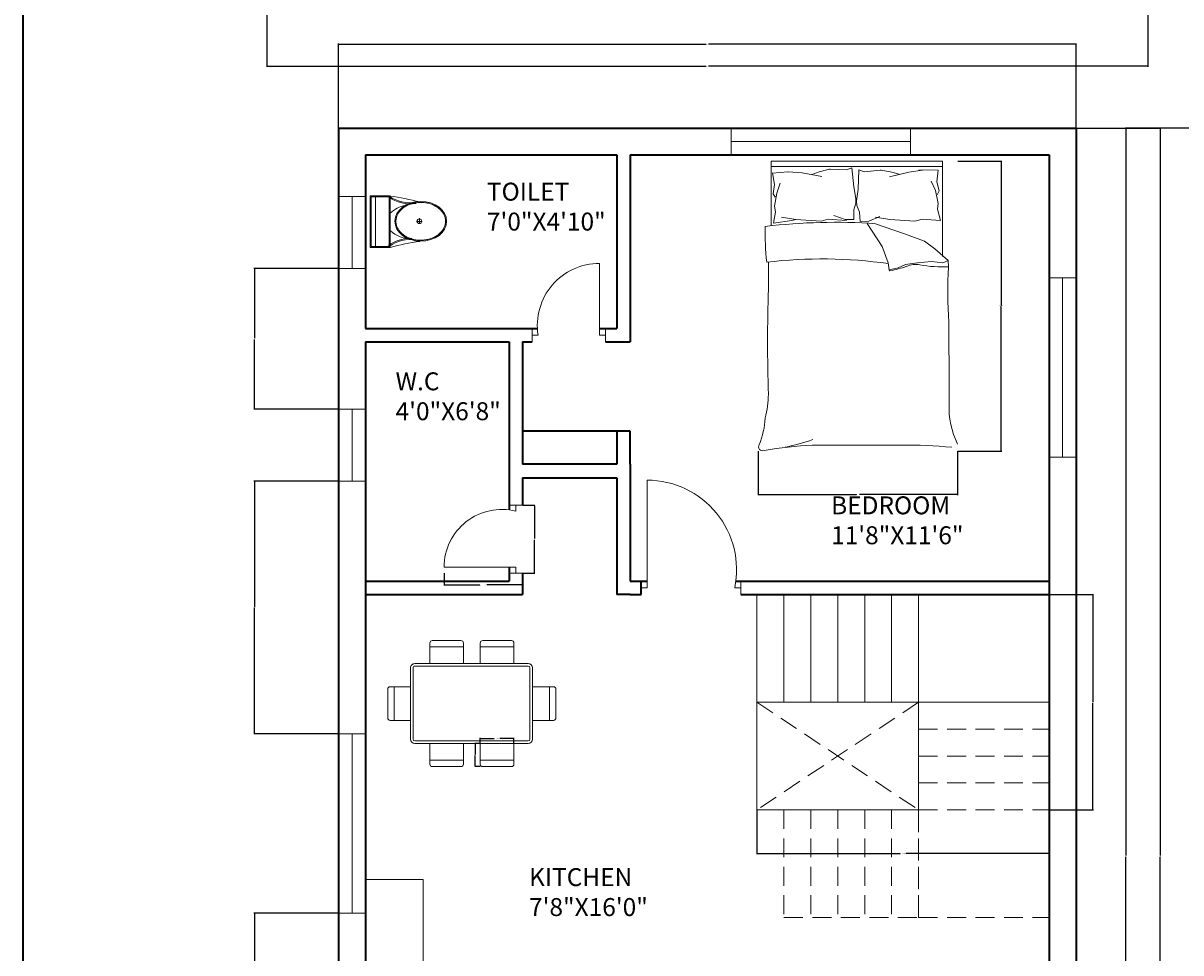
# Model space of a CAD drawing. Units: inches. Extents: x 1911 to 3278, y 2022 to 3108.
# Tile 8 of 13: x 1911 to 2298, y 2345 to 2656. Entities that reach past the tile are written whole.
import ezdxf

# ---------------------------------------------------------------- set-up
doc = ezdxf.new("R2010")
doc.units = ezdxf.units.IN
doc.linetypes.add('DASHED2', pattern=[9.525, 6.35, -3.175])
for name, color, linetype, lineweight in [('A-ANNO-DIMS', 2, 'Continuous', 18), ('A-ANNO-TTLB', 7, 'Continuous', 35), ('A-AREA-IDEN', 7, 'Continuous', 18), ('A-DOOR', 4, 'Continuous', 18), ('A-FLOR-CASE', 9, 'Continuous', 18), ('A-FLOR-FIXT', 9, 'Continuous', 18), ('A-FLOR-STRS', 7, 'Continuous', 18), ('A-FLOR-STRS-OVHD', 253, 'DASHED2', 13), ('A-FURN', 8, 'Continuous', 13), ('A-GLAZ', 4, 'Continuous', 18), ('A-WALL', 7, 'Continuous', 35)]:
    doc.layers.add(name, color=color, linetype=linetype, lineweight=lineweight)
doc.styles.get("Standard").update_dxf_attribs({"font": 'arial.ttf'})
doc.dimstyles.get("Standard").update_dxf_attribs({"dimtxt": 0.18, "dimasz": 0.18, "dimexe": 0.18, "dimexo": 0.0625, "dimgap": 0.09, "dimtad": 0, "dimtih": 1, "dimtoh": 1, "dimdec": 4, "dimzin": 0, "dimdsep": 46, "dimtxsty": 'Standard', "dimcen": 0.09, "dimadec": 0, "dimazin": 0, "dimtfac": 1, "dimtdec": 4, "dimtofl": 0, "dimtmove": 0, "dimatfit": 3, "dimfxl": 1, "dimtolj": 1, "dimtzin": 0, "dimarcsym": 0})

# ---------------------------------------------------------------- blocks, each defined once
blk = doc.blocks.new('A$C31115884')
for p, q in [((283, 498), (223, 498)), ((258, 466), (258, 523)), ((0, 200), (0, 0)), ((520, 200), (0, 200)), ((10, 190), (10, 10)), ((510, 190), (10, 190)), ((510, 10), (510, 190)), ((520, 0), (520, 200)), ((510, 54), (0, 54)), ((10, 10), (510, 10)), ((0, 0), (520, 0))]:
    blk.add_line(p, q)
blk.add_circle((256, 496), 23.6)
for centre, radius, start, end in [((2778, -205), 2807, 165.4549, 171.7133), ((3237, 905), 2807, 188.2867, 194.5451), ((-295, 403), 365, 324.2091, 9.3499), ((-295, 403), 375, 324.2091, 9.3499), ((384, 406), 293, 190.2774, 224.1564), ((139, 406), 293, 315.8436, 2.6563), ((806, 403), 375, 179.2036, 215.7909), ((806, 403), 365, 170.6501, 215.7909)]:
    blk.add_arc(centre, radius, start, end)
blk.add_ellipse((256, 510), major_axis=(0, -261), ratio=0.772727)
blk.add_open_spline([(256, 259), (263, 259), (270, 260), (288, 262), (299, 265), (320, 273), (330, 278), (350, 291), (360, 299), (378, 316), (386, 326), (402, 347), (409, 358), (421, 383), (427, 395), (436, 422), (440, 436), (445, 465), (447, 480), (448, 509), (448, 524), (445, 553), (443, 568), (436, 596), (432, 610), (422, 636), (416, 649), (402, 672), (395, 683), (379, 703), (370, 712), (351, 728), (341, 735), (321, 746), (310, 751), (289, 757), (278, 759), (256, 761), (245, 761), (223, 757), (212, 754), (191, 746), (181, 741), (161, 728), (151, 720), (133, 703), (125, 693), (110, 672), (103, 660), (90, 636), (85, 623), (76, 596), (72, 582), (67, 553), (66, 538), (64, 509), (65, 494), (68, 465), (70, 450), (77, 422), (81, 408), (91, 382), (97, 370), (111, 346), (118, 335), (135, 316), (144, 307), (162, 291), (172, 284), (193, 273), (203, 269), (225, 262), (236, 260), (250, 259), (253, 259), (256, 259)], degree=3, knots=[0, 0, 0, 0, 0.110105, 0.110105, 0.285049, 0.285049, 0.459994, 0.459994, 0.634938, 0.634938, 0.809882, 0.809882, 0.984827, 0.984827, 1.159771, 1.159771, 1.334715, 1.334715, 1.50966, 1.50966, 1.684604, 1.684604, 1.859549, 1.859549, 2.034493, 2.034493, 2.209437, 2.209437, 2.384382, 2.384382, 2.559326, 2.559326, 2.73427, 2.73427, 2.909215, 2.909215, 3.084159, 3.084159, 3.259103, 3.259103, 3.434048, 3.434048, 3.608992, 3.608992, 3.783936, 3.783936, 3.958881, 3.958881, 4.133825, 4.133825, 4.30877, 4.30877, 4.483714, 4.483714, 4.658658, 4.658658, 4.833603, 4.833603, 5.008547, 5.008547, 5.183491, 5.183491, 5.358436, 5.358436, 5.53338, 5.53338, 5.708324, 5.708324, 5.883269, 5.883269, 6.058213, 6.058213, 6.233158, 6.233158, 6.283185, 6.283185, 6.283185, 6.283185])
blk = doc.blocks.new('WIN-60')
for p, q in [((0, 60), (9, 60)), ((9, 60), (4.5, 60)), ((4.5, 60), (4.5, 0)), ((4.5, 0), (0, 0)), ((0, 0), (9, 0))]:
    blk.add_line(p, q)
blk = doc.blocks.new('WIN-24')
for p, q in [((0, 24), (9, 24)), ((9, 24), (4.5, 24)), ((4.5, 24), (4.5, 0)), ((4.5, 0), (0, 0)), ((0, 0), (9, 0))]:
    blk.add_line(p, q)
blk = doc.blocks.new('WIN-24-ALT-JAMB')
for p, q in [((0, 24), (9, 24)), ((9, 24), (4.5, 24)), ((4.5, 24), (4.5, 0)), ((9, 0), (0, 0)), ((4.5, 0), (9, 0))]:
    blk.add_line(p, q)
blk = doc.blocks.new('DOOR-BATH-GF')
for p, q in [((22.54, 2.25), (22.54, 26.25)), ((0, 4.5), (0, 0)), ((24.54, 0), (24.54, 4.5)), ((24.54, 4.5), (24.54, 2.25)), ((0, 0), (0, 2.25)), ((0, 2.25), (2, 2.25)), ((24.54, 2.25), (22.54, 2.25))]:
    blk.add_line(p, q)
blk.add_arc((22.54, 5.46), 20.79, 90, 188.8739)
blk = doc.blocks.new('DOOR-WC-GF')
for p, q in [((21.75, 22.69), (26.25, 22.69)), ((26.25, 22.69), (24, 22.69)), ((24, 22.69), (24, 20.69)), ((24, 2), (0, 2)), ((24, 0), (24, 2)), ((21.75, 0), (26.25, 0)), ((26.25, 0), (24, 0))]:
    blk.add_line(p, q)
blk.add_arc((19.28, 2), 19.28, 75.8267, 180)
blk = doc.blocks.new('DOOR-BED-GF')
for p, q in [((2, 2.25), (2, 38.25)), ((0, 4.5), (0, 0)), ((33.28, 4.5), (33.28, 0)), ((0, 0), (0, 2.25)), ((0, 2.25), (0, 2.25)), ((0, 2.25), (2, 2.25)), ((33.28, 2.25), (31.28, 2.25)), ((33.28, 0), (33.28, 2.25))]:
    blk.add_line(p, q)
blk.add_arc((2, 8.34), 29.91, 348.2504, 90)
blk = doc.blocks.new('BED-DOUBLE')
for p, q in [((4.17, 75.16), (4.17, 96.87)), ((4.17, 96.87), (61.46, 96.87)), ((61.46, 96.87), (61.46, 64.97)), ((4.17, 95.03), (61.46, 95.03)), ((4.67, 92.87), (9.81, 93.27)), ((4.67, 92.9), (5.36, 89.08)), ((9.81, 93.27), (9.93, 93.24)), ((9.93, 93.24), (14.52, 92.9)), ((14.52, 92.9), (21.1, 91.68)), ((17.81, 92.38), (20.24, 93.24)), ((20.24, 93.24), (23.7, 94.11)), ((23.7, 94.11), (24.09, 94.11)), ((24.09, 94.11), (29.42, 93.94)), ((29.42, 93.94), (31.15, 94.63)), ((31.15, 94.63), (31.84, 88.22)), ((33.54, 93.88), (33.25, 87.44)), ((35.31, 93.3), (33.54, 93.88)), ((40.62, 93.81), (35.31, 93.3)), ((41.01, 93.83), (40.62, 93.81)), ((44.52, 93.18), (41.01, 93.83)), ((50.25, 93.19), (43.75, 91.57)), ((47, 92.47), (44.52, 93.18)), ((54.8, 93.82), (50.25, 93.19)), ((60.08, 93.81), (53.6, 93.92)), ((53.6, 93.92), (54.8, 93.82)), ((60.08, 93.81), (59.62, 89.96)), ((5.36, 89.08), (4.84, 85.96)), ((6.06, 86.14), (7.27, 89.43)), ((59.12, 86.97), (57.7, 90.18)), ((59.62, 89.96), (60.34, 86.88)), ((4.84, 85.96), (5.54, 84.75)), ((5.36, 81.8), (6.06, 86.14)), ((31.84, 88.22), (32.54, 84.4)), ((33.25, 87.44), (32.79, 83.59)), ((60.08, 82.69), (59.12, 86.97)), ((60.34, 86.88), (59.72, 85.62)), ((5.71, 79.9), (5.36, 81.8)), ((32.54, 82.84), (31.84, 80.59)), ((32.54, 84.4), (32.54, 82.84)), ((32.79, 83.59), (32.89, 82.03)), ((32.89, 82.03), (33.72, 79.83)), ((59.85, 80.77), (60.08, 82.69)), ((5.02, 76.08), (5.71, 79.9)), ((7.65, 78.14), (12.48, 77.34)), ((20.89, 76.82), (23.24, 77.49)), ((23.24, 77.49), (29.39, 77)), ((28.9, 77.37), (25.13, 78.68)), ((31.84, 80.59), (31.84, 77.37)), ((33.72, 79.83), (33.93, 76.62)), ((36.87, 76.8), (40.55, 78.34)), ((39.04, 78.14), (43.87, 77.34)), ((52.28, 76.82), (54.63, 77.49)), ((54.63, 77.49), (60.78, 77)), ((60.78, 77), (59.85, 80.77)), ((11.13, 76.95), (5.02, 76.08)), ((12.48, 77.34), (11.13, 76.95)), ((12.48, 77.34), (20.89, 76.82)), ((31.84, 77.37), (28.9, 77.37)), ((33.93, 76.62), (36.87, 76.8)), ((36.28, 76.03), (41.3, 68.25)), ((48.73, 72.52), (38.73, 76.03)), ((43.87, 77.34), (52.28, 76.82)), ((55.41, 70.1), (48.73, 72.52)), ((58.94, 67.51), (55.41, 70.1)), ((41.3, 68.25), (43.34, 62.87)), ((63.38, 63.61), (58.94, 67.51)), ((43.34, 62.87), (43.71, 60.45)), ((46.68, 61.2), (49.1, 62.31)), ((49.1, 62.31), (53.18, 62.87)), ((53.18, 62.87), (57.82, 63.24)), ((57.82, 63.24), (61.54, 62.87)), ((61.54, 62.87), (63.38, 63.61)), ((63.48, 61.52), (63.38, 63.61, 4.64)), ((43.71, 60.45), (46.68, 61.2)), ((18.06, 1.87), (47.57, 1.87))]:
    blk.add_line(p, q)
for centre, radius, start, end in [((102.1, 72.78), 99.87, 178.7218, 185.604), ((25.61, -121.38), 197.77, 86.0865, 96.7821), ((21.29, -90.53), 154.68, 81.7845, 96.9006), ((-200.58, 59.5), 203.94, 358.4762, 1.0082), ((52.44, 54.83), 7.46, 78.6608, 113.7384), ((61.53, 104.85), 43.38, 259.8763, 272.5657), ((43.92, 60.38), 0.221, 160.2464, 271.1377), ((37.35, 95.1), 35.55, 280.6617, 289.8806), ((218.51, 53.34), 155.25, 176.9791, 183.8365), ((581.23, 36.19), 578.22, 178.22771, 181.71854), ((-5405.34, 15.56), 5469.02, 0.00217, 0.28689), ((-32.25, 19.53), 35.53, 346.0648, 358.9113), ((91.3, 14.55), 27.65, 177.4714, 206.4681), ((-25.97, 12.62), 28.25, 337.9751, 356.652), ((1.3, 1.3), 1.31, 146.1736, 293.4781), ((25.69, -143.9), 145.97, 92.9958, 99.4091), ((-20.65, 125.3), 127.63, 283.3832, 287.7053), ((49.34, -157.62), 159.5, 84.4998, 90.6351)]:
    blk.add_arc(centre, radius, start, end)
blk = doc.blocks.new('CHAIR-DINING')
for p, q in [((0, 0), (0, 6.88)), ((11.24, 5.62), (0, 5.62)), ((0.84, 7.73), (10.4, 7.73)), ((11.24, 6.88), (11.24, 0))]:
    blk.add_line(p, q)
for centre, start, end in [((0.84, 6.88), 90, 180), ((10.4, 6.88), 0, 90)]:
    blk.add_arc(centre, 0.843, start, end)
blk = doc.blocks.new('COUNTER-KITCHEN-L')
for p, q in [((19.27, 79.32), (0, 79.32)), ((19.27, 0), (19.27, 79.32)), ((92, 0), (19.27, 0))]:
    blk.add_line(p, q)
blk = doc.blocks.new('STAIR-PLAN-GF')
for p, q in [((0, 36), (0, 72)), ((9, 36), (9, 72)), ((18, 36), (18, 72)), ((27, 36), (27, 72)), ((36, 36), (36, 72)), ((45, 36), (45, 72)), ((54, 36), (54, 72)), ((28.63, 36), (0, 36)), ((0, 36), (0, 0)), ((28.63, 36), (97.65, 36)), ((54, 36), (54, 0)), ((54, 36), (54, 27)), ((0, 0), (48, 0)), ((54, 0), (48, 0))]:
    blk.add_line(p, q)
blk = doc.blocks.new('STAIR-BEYOND-GF')
for p, q in [((54, 72), (0, 36)), ((0, 72), (54, 36)), ((54, 72), (54, 63)), ((54, 63), (97.65, 63)), ((54, 54), (97.65, 54)), ((54, 45), (97.65, 45)), ((9, 36), (9, 0)), ((18, 36), (18, 0)), ((27, 36), (27, 0)), ((36, 36), (36, 0)), ((45, 36), (45, 0)), ((54, 36), (97.65, 36)), ((54, 0), (54, 36)), ((54, 36), (54, 0)), ((9, 0), (54, 0)), ((54, 0), (97.65, 0))]:
    blk.add_line(p, q)
blk = doc.blocks.new('*D32')
at = {"layer": 'A-ANNO-DIMS', "color": 0, "lineweight": -2, "transparency": 16777216}
for p, q in [((2064.18, 2415.14), (2064.18, 2416.95)), ((2064.36, 2416.77), (2068.85, 2416.77)), ((2075.24, 2416.77), (2070.75, 2416.77)), ((2075.42, 2415.14), (2075.42, 2416.95))]:
    blk.add_line(p, q, dxfattribs=at)
at = {"layer": 'A-ANNO-DIMS', "color": 0, "transparency": 16777216}
for points in [[(2064.36, 2416.8), (2064.36, 2416.74), (2064.18, 2416.77)], [(2075.24, 2416.8), (2075.24, 2416.74), (2075.42, 2416.77)]]:
    blk.add_solid(points, dxfattribs=at)
at = {"layer": 'Defpoints', "color": 0, "transparency": 16777216}
for p in [(2064.18, 2416.77), (2064.18, 2415.08), (2075.42, 2415.08)]:
    blk.add_point(p, dxfattribs=at)
at = {"layer": 'A-ANNO-DIMS', "color": 0, "transparency": 16777216, "insert": (2069.8, 2416.77), "char_height": 0.18, "attachment_point": 5}
blk.add_mtext('\\A1;CHAIR 11 TYP.', dxfattribs=at)
blk = doc.blocks.new('*D33')
at = {"layer": 'A-ANNO-DIMS', "color": 0, "lineweight": -2, "transparency": 16777216}
for p, q in [((2064.12, 2415.08), (2062.32, 2415.08)), ((2062.5, 2414.9), (2062.5, 2411.4)), ((2062.5, 2407.53), (2062.5, 2411.03)), ((2064.12, 2407.35), (2062.32, 2407.35))]:
    blk.add_line(p, q, dxfattribs=at)
at = {"layer": 'A-ANNO-DIMS', "color": 0, "transparency": 16777216}
for points in [[(2062.47, 2414.9), (2062.53, 2414.9), (2062.5, 2415.08)], [(2062.47, 2407.53), (2062.53, 2407.53), (2062.5, 2407.35)]]:
    blk.add_solid(points, dxfattribs=at)
at = {"layer": 'Defpoints', "color": 0, "transparency": 16777216}
for p in [(2064.18, 2415.08), (2062.5, 2407.35), (2064.18, 2407.35)]:
    blk.add_point(p, dxfattribs=at)
at = {"layer": 'A-ANNO-DIMS', "color": 0, "transparency": 16777216, "insert": (2062.5, 2411.22), "char_height": 0.18, "attachment_point": 5}
blk.add_mtext('\\A1;8 TYP.', dxfattribs=at)
blk = doc.blocks.new('*D36')
at = {"layer": 'A-ANNO-DIMS', "color": 0, "lineweight": -2, "transparency": 16777216}
for p, q in [((2223.83, 2609.84), (2238.5, 2609.84)), ((2238.32, 2609.66), (2238.32, 2561.52)), ((2238.32, 2513.02), (2238.32, 2561.16)), ((2223.83, 2512.84), (2238.5, 2512.84))]:
    blk.add_line(p, q, dxfattribs=at)
at = {"layer": 'A-ANNO-DIMS', "color": 0, "transparency": 16777216}
for points in [[(2238.29, 2609.66), (2238.35, 2609.66), (2238.32, 2609.84)], [(2238.29, 2513.02), (2238.35, 2513.02), (2238.32, 2512.84)]]:
    blk.add_solid(points, dxfattribs=at)
at = {"layer": 'Defpoints', "color": 0, "transparency": 16777216}
for p in [(2223.77, 2609.84), (2238.32, 2609.84), (2223.77, 2512.84)]:
    blk.add_point(p, dxfattribs=at)
at = {"layer": 'A-ANNO-DIMS', "color": 0, "transparency": 16777216, "insert": (2238.32, 2561.34), "char_height": 0.18, "attachment_point": 5}
blk.add_mtext('\\A1;BED 97 TYP.', dxfattribs=at)
blk = doc.blocks.new('*D37')
at = {"layer": 'A-ANNO-DIMS', "color": 0, "lineweight": -2, "transparency": 16777216}
for p, q in [((2157.12, 2512.78), (2157.12, 2498.11)), ((2223.77, 2512.78), (2223.77, 2498.11)), ((2157.3, 2498.29), (2189.91, 2498.29)), ((2223.59, 2498.29), (2190.97, 2498.29))]:
    blk.add_line(p, q, dxfattribs=at)
at = {"layer": 'A-ANNO-DIMS', "color": 0, "transparency": 16777216}
for points in [[(2157.3, 2498.32), (2157.3, 2498.26), (2157.12, 2498.29)], [(2223.59, 2498.32), (2223.59, 2498.26), (2223.77, 2498.29)]]:
    blk.add_solid(points, dxfattribs=at)
at = {"layer": 'Defpoints', "color": 0, "transparency": 16777216}
for p in [(2157.12, 2512.84), (2223.77, 2512.84), (2223.77, 2498.29)]:
    blk.add_point(p, dxfattribs=at)
at = {"layer": 'A-ANNO-DIMS', "color": 0, "transparency": 16777216, "insert": (2190.44, 2498.29), "char_height": 0.18, "attachment_point": 5}
blk.add_mtext('\\A1;67 TYP.', dxfattribs=at)
blk = doc.blocks.new('*D40')
at = {"layer": 'A-ANNO-DIMS', "color": 0, "lineweight": -2, "transparency": 16777216}
for p, q in [((2052.08, 2471.98), (2052.08, 2467.92)), ((2078.33, 2471.98), (2078.33, 2467.92)), ((2052.26, 2468.1), (2064.02, 2468.1)), ((2078.15, 2468.1), (2066.4, 2468.1))]:
    blk.add_line(p, q, dxfattribs=at)
at = {"layer": 'A-ANNO-DIMS', "color": 0, "transparency": 16777216}
for points in [[(2052.26, 2468.13), (2052.26, 2468.07), (2052.08, 2468.1)], [(2078.15, 2468.13), (2078.15, 2468.07), (2078.33, 2468.1)]]:
    blk.add_solid(points, dxfattribs=at)
at = {"layer": 'Defpoints', "color": 0, "transparency": 16777216}
for p in [(2052.08, 2472.04), (2078.33, 2472.04), (2078.33, 2468.1)]:
    blk.add_point(p, dxfattribs=at)
at = {"layer": 'A-ANNO-DIMS', "color": 0, "transparency": 16777216, "insert": (2065.21, 2468.1), "char_height": 0.18, "attachment_point": 5}
blk.add_mtext('\\A1;WC DOOR 26 TYP.', dxfattribs=at)
blk = doc.blocks.new('*D41')
at = {"layer": 'A-ANNO-DIMS', "color": 0, "lineweight": -2, "transparency": 16777216}
for p, q in [((2078.4, 2494.73), (2082.45, 2494.73)), ((2082.27, 2494.55), (2082.27, 2483.57)), ((2082.27, 2472.22), (2082.27, 2483.2)), ((2078.4, 2472.04), (2082.45, 2472.04))]:
    blk.add_line(p, q, dxfattribs=at)
at = {"layer": 'A-ANNO-DIMS', "color": 0, "transparency": 16777216}
for points in [[(2082.24, 2494.55), (2082.3, 2494.55), (2082.27, 2494.73)], [(2082.24, 2472.22), (2082.3, 2472.22), (2082.27, 2472.04)]]:
    blk.add_solid(points, dxfattribs=at)
at = {"layer": 'Defpoints', "color": 0, "transparency": 16777216}
for p in [(2078.33, 2494.73), (2082.27, 2494.73), (2078.33, 2472.04)]:
    blk.add_point(p, dxfattribs=at)
at = {"layer": 'A-ANNO-DIMS', "color": 0, "transparency": 16777216, "insert": (2082.27, 2483.39), "char_height": 0.18, "attachment_point": 5}
blk.add_mtext('\\A1;23 TYP.', dxfattribs=at)
blk = doc.blocks.new('*D60')
at = {"layer": 'A-ANNO-DIMS', "color": 0, "lineweight": -2, "transparency": 16777216}
for p, q in [((2156.69, 2392.81), (2156.69, 2378.05)), ((2254.33, 2392.81), (2254.33, 2378.05)), ((2156.87, 2378.23), (2204.58, 2378.23)), ((2254.15, 2378.23), (2206.44, 2378.23))]:
    blk.add_line(p, q, dxfattribs=at)
at = {"layer": 'A-ANNO-DIMS', "color": 0, "transparency": 16777216}
for points in [[(2156.87, 2378.26), (2156.87, 2378.2), (2156.69, 2378.23)], [(2254.15, 2378.26), (2254.15, 2378.2), (2254.33, 2378.23)]]:
    blk.add_solid(points, dxfattribs=at)
at = {"layer": 'Defpoints', "color": 0, "transparency": 16777216}
for p in [(2156.69, 2392.87), (2254.33, 2392.87), (2254.33, 2378.23)]:
    blk.add_point(p, dxfattribs=at)
at = {"layer": 'A-ANNO-DIMS', "color": 0, "transparency": 16777216, "insert": (2205.51, 2378.23), "char_height": 0.18, "attachment_point": 5}
blk.add_mtext('\\A1;STAIR 98 TYP.', dxfattribs=at)
blk = doc.blocks.new('*D61')
at = {"layer": 'A-ANNO-DIMS', "color": 0, "lineweight": -2, "transparency": 16777216}
for p, q in [((2254.4, 2464.87), (2269.16, 2464.87)), ((2268.98, 2464.69), (2268.98, 2429.05)), ((2268.98, 2393.05), (2268.98, 2428.69)), ((2254.4, 2392.87), (2269.16, 2392.87))]:
    blk.add_line(p, q, dxfattribs=at)
at = {"layer": 'A-ANNO-DIMS', "color": 0, "transparency": 16777216}
for points in [[(2268.95, 2464.69), (2269.01, 2464.69), (2268.98, 2464.87)], [(2268.95, 2393.05), (2269.01, 2393.05), (2268.98, 2392.87)]]:
    blk.add_solid(points, dxfattribs=at)
at = {"layer": 'Defpoints', "color": 0, "transparency": 16777216}
for p in [(2254.33, 2464.87), (2268.98, 2464.87), (2254.33, 2392.87)]:
    blk.add_point(p, dxfattribs=at)
at = {"layer": 'A-ANNO-DIMS', "color": 0, "transparency": 16777216, "insert": (2268.98, 2428.87), "char_height": 0.18, "attachment_point": 5}
blk.add_mtext('\\A1;72 TYP.', dxfattribs=at)
blk = doc.blocks.new('*D66')
at = {"layer": 'A-ANNO-DIMS', "color": 0, "lineweight": -2, "transparency": 16777216}
for p, q in [((2016.83, 2620.94), (2016.83, 2649.15)), ((2017.01, 2648.97), (2139.69, 2648.97)), ((2263.15, 2648.97), (2140.48, 2648.97)), ((2263.33, 2620.94), (2263.33, 2649.15))]:
    blk.add_line(p, q, dxfattribs=at)
at = {"layer": 'A-ANNO-DIMS', "color": 0, "transparency": 16777216}
for points in [[(2017.01, 2649), (2017.01, 2648.94), (2016.83, 2648.97)], [(2263.15, 2649), (2263.15, 2648.94), (2263.33, 2648.97)]]:
    blk.add_solid(points, dxfattribs=at)
at = {"layer": 'Defpoints', "color": 0, "transparency": 16777216}
for p in [(2263.33, 2648.97), (2016.83, 2620.87), (2263.33, 2620.87)]:
    blk.add_point(p, dxfattribs=at)
at = {"layer": 'A-ANNO-DIMS', "color": 0, "transparency": 16777216, "insert": (2140.08, 2648.97), "char_height": 0.18, "attachment_point": 5}
blk.add_mtext('\\A1;246.5', dxfattribs=at)
blk = doc.blocks.new('*D67')
at = {"layer": 'A-ANNO-DIMS', "color": 0, "lineweight": -2, "transparency": 16777216}
for p, q in [((2263.4, 2620.87), (2291.61, 2620.87)), ((2291.43, 2620.69), (2291.43, 2377.56)), ((2291.43, 2134.05), (2291.43, 2377.19)), ((2263.4, 2133.87), (2291.61, 2133.87))]:
    blk.add_line(p, q, dxfattribs=at)
at = {"layer": 'A-ANNO-DIMS', "color": 0, "transparency": 16777216}
for points in [[(2291.4, 2620.69), (2291.46, 2620.69), (2291.43, 2620.87)], [(2291.4, 2134.05), (2291.46, 2134.05), (2291.43, 2133.87)]]:
    blk.add_solid(points, dxfattribs=at)
at = {"layer": 'Defpoints', "color": 0, "transparency": 16777216}
for p in [(2263.33, 2620.87), (2291.43, 2620.87), (2263.33, 2133.87)]:
    blk.add_point(p, dxfattribs=at)
at = {"layer": 'A-ANNO-DIMS', "color": 0, "transparency": 16777216, "insert": (2291.43, 2377.37), "char_height": 0.18, "attachment_point": 5}
blk.add_mtext('\\A1;487', dxfattribs=at)
blk = doc.blocks.new('*D72')
at = {"layer": 'A-ANNO-DIMS', "color": 0, "lineweight": -2, "transparency": 16777216}
for p, q in [((2016.77, 2358.3), (1988.55, 2358.3)), ((1988.73, 2358.12), (1988.73, 2311.27)), ((1988.73, 2264.05), (1988.73, 2310.9)), ((2016.77, 2263.87), (1988.55, 2263.87))]:
    blk.add_line(p, q, dxfattribs=at)
at = {"layer": 'A-ANNO-DIMS', "color": 0, "transparency": 16777216}
for points in [[(1988.7, 2358.12), (1988.76, 2358.12), (1988.73, 2358.3)], [(1988.7, 2264.05), (1988.76, 2264.05), (1988.73, 2263.87)]]:
    blk.add_solid(points, dxfattribs=at)
at = {"layer": 'Defpoints', "color": 0, "transparency": 16777216}
for p in [(1988.73, 2358.3), (2016.83, 2358.3), (2016.83, 2263.87)]:
    blk.add_point(p, dxfattribs=at)
at = {"layer": 'A-ANNO-DIMS', "color": 0, "transparency": 16777216, "insert": (1988.73, 2311.09), "char_height": 0.18, "attachment_point": 5}
blk.add_mtext('\\A1;94.43', dxfattribs=at)
blk = doc.blocks.new('*D73')
at = {"layer": 'A-ANNO-DIMS', "color": 0, "lineweight": -2, "transparency": 16777216}
for p, q in [((2016.77, 2502.84), (1988.55, 2502.84)), ((1988.73, 2502.66), (1988.73, 2460.75)), ((1988.73, 2418.48), (1988.73, 2460.39)), ((2016.77, 2418.3), (1988.55, 2418.3))]:
    blk.add_line(p, q, dxfattribs=at)
at = {"layer": 'A-ANNO-DIMS', "color": 0, "transparency": 16777216}
for points in [[(1988.7, 2502.66), (1988.76, 2502.66), (1988.73, 2502.84)], [(1988.7, 2418.48), (1988.76, 2418.48), (1988.73, 2418.3)]]:
    blk.add_solid(points, dxfattribs=at)
at = {"layer": 'Defpoints', "color": 0, "transparency": 16777216}
for p in [(1988.73, 2502.84), (2016.83, 2502.84), (2016.83, 2418.3)]:
    blk.add_point(p, dxfattribs=at)
at = {"layer": 'A-ANNO-DIMS', "color": 0, "transparency": 16777216, "insert": (1988.73, 2460.57), "char_height": 0.18, "attachment_point": 5}
blk.add_mtext('\\A1;84.54', dxfattribs=at)
blk = doc.blocks.new('*D74')
at = {"layer": 'A-ANNO-DIMS', "color": 0, "lineweight": -2, "transparency": 16777216}
for p, q in [((2016.77, 2573.94), (1988.55, 2573.94)), ((1988.73, 2573.76), (1988.73, 2550.57)), ((1988.73, 2527.02), (1988.73, 2550.21)), ((2016.77, 2526.84), (1988.55, 2526.84))]:
    blk.add_line(p, q, dxfattribs=at)
at = {"layer": 'A-ANNO-DIMS', "color": 0, "transparency": 16777216}
for points in [[(1988.7, 2573.76), (1988.76, 2573.76), (1988.73, 2573.94)], [(1988.7, 2527.02), (1988.76, 2527.02), (1988.73, 2526.84)]]:
    blk.add_solid(points, dxfattribs=at)
at = {"layer": 'Defpoints', "color": 0, "transparency": 16777216}
for p in [(1988.73, 2573.94), (2016.83, 2573.94), (2016.83, 2526.84)]:
    blk.add_point(p, dxfattribs=at)
at = {"layer": 'A-ANNO-DIMS', "color": 0, "transparency": 16777216, "insert": (1988.73, 2550.39), "char_height": 0.18, "attachment_point": 5}
blk.add_mtext('\\A1;47.1', dxfattribs=at)
blk = doc.blocks.new('*D76')
at = {"layer": 'A-ANNO-DIMS', "color": 0, "lineweight": -2, "transparency": 16777216}
for p, q in [((2308.06, 2620.87), (2279.84, 2620.87)), ((2280.02, 2620.69), (2280.02, 2377.56)), ((2280.02, 2134.05), (2280.02, 2377.19)), ((2308.06, 2133.87), (2279.84, 2133.87))]:
    blk.add_line(p, q, dxfattribs=at)
at = {"layer": 'A-ANNO-DIMS', "color": 0, "transparency": 16777216}
for points in [[(2279.99, 2620.69), (2280.05, 2620.69), (2280.02, 2620.87)], [(2279.99, 2134.05), (2280.05, 2134.05), (2280.02, 2133.87)]]:
    blk.add_solid(points, dxfattribs=at)
at = {"layer": 'Defpoints', "color": 0, "transparency": 16777216}
for p in [(2280.02, 2620.87), (2308.12, 2620.87), (2308.12, 2133.87)]:
    blk.add_point(p, dxfattribs=at)
at = {"layer": 'A-ANNO-DIMS', "color": 0, "transparency": 16777216, "insert": (2280.02, 2377.37), "char_height": 0.18, "attachment_point": 5}
blk.add_mtext('\\A1;487', dxfattribs=at)
blk = doc.blocks.new('*D89')
at = {"layer": 'A-ANNO-DIMS', "color": 0, "lineweight": -2, "transparency": 16777216}
for p, q in [((1992.83, 2841.96), (1992.83, 2641.37)), ((2287.33, 2841.96), (2287.33, 2641.37)), ((1993.01, 2641.55), (2139.69, 2641.55)), ((2287.15, 2641.55), (2140.48, 2641.55))]:
    blk.add_line(p, q, dxfattribs=at)
at = {"layer": 'A-ANNO-DIMS', "color": 0, "transparency": 16777216}
for points in [[(1993.01, 2641.58), (1993.01, 2641.52), (1992.83, 2641.55)], [(2287.15, 2641.58), (2287.15, 2641.52), (2287.33, 2641.55)]]:
    blk.add_solid(points, dxfattribs=at)
at = {"layer": 'Defpoints', "color": 0, "transparency": 16777216}
for p in [(1992.83, 2842.03), (2287.33, 2842.03), (2287.33, 2641.55)]:
    blk.add_point(p, dxfattribs=at)
at = {"layer": 'A-ANNO-DIMS', "color": 0, "transparency": 16777216, "insert": (2140.08, 2641.55), "char_height": 0.18, "attachment_point": 5}
blk.add_mtext('\\A1;294.5', dxfattribs=at)

msp = doc.modelspace()

# ---------------------------------------------------------------- linework, layer by layer
at = {"layer": 'A-ANNO-TTLB'}
msp.add_lwpolyline([(1911.3875, 3108.0628), (3278.3142, 3108.0628), (3278.3142, 2021.7237), (1911.3875, 2021.7237)], close=True, dxfattribs=at)
at = {"layer": 'A-FURN'}
for p, q in [((2040.8627, 2416.4843), (2040.8627, 2440.366)), ((2041.7056, 2416.4843), (2041.7056, 2440.366)), ((2042.2674, 2441.7709), (2080.1973, 2441.7709)), ((2042.2674, 2440.928), (2080.1973, 2440.928)), ((2080.7592, 2440.366), (2080.7592, 2416.4843)), ((2081.6021, 2440.366), (2081.6021, 2416.4843)), ((2033.2767, 2433.2015), (2033.2767, 2423.6488)), ((2040.8627, 2434.0444), (2034.1196, 2434.0444)), ((2035.3839, 2422.8059), (2035.3839, 2434.0444)), ((2081.6021, 2434.0444), (2088.6261, 2434.0444)), ((2087.3618, 2422.8059), (2087.3618, 2434.0444)), ((2089.469, 2433.2015), (2089.469, 2423.6488)), ((2034.1196, 2422.8059), (2040.8627, 2422.8059)), ((2088.6261, 2422.8059), (2081.6021, 2422.8059)), ((2080.1973, 2415.9224), (2042.2674, 2415.9224)), ((2080.1973, 2415.0795), (2042.2674, 2415.0795))]:
    msp.add_line(p, q, dxfattribs=at)
for centre, radius, start, end in [((2042.2674, 2440.366), 1.4048, 90, 180.00001), ((2042.2674, 2440.366), 0.5619, 90, 180.00001), ((2080.1973, 2440.366), 1.4048, 0, 90), ((2080.1973, 2440.366), 0.5619, 0, 90), ((2034.1196, 2433.2015), 0.8429, 90, 180), ((2088.6261, 2433.2015), 0.8429, 0, 90), ((2034.1196, 2423.6488), 0.8429, 180, 270), ((2088.6261, 2423.6488), 0.8429, 270, 0), ((2042.2674, 2416.4843), 1.4048, 180.000003, 270), ((2042.2674, 2416.4843), 0.5619, 180.000003, 270), ((2080.1973, 2416.4843), 1.4048, 270, 0), ((2080.1973, 2416.4843), 0.5619, 270, 0)]:
    msp.add_arc(centre, radius, start, end, dxfattribs=at)
at = {"layer": 'A-WALL'}
for p, q in [((2016.8344, 2620.8733), (2016.8344, 2133.8733)), ((2016.8344, 2620.8733), (2016.8344, 2133.8733)), ((2016.8344, 2620.8733), (2263.3344, 2620.8733)), ((2263.3344, 2620.8733), (2263.3344, 2133.8733)), ((2025.8344, 2611.8733), (2109.8344, 2611.8733)), ((2025.8344, 2611.8733), (2025.8344, 2553.8733)), ((2109.8344, 2611.8733), (2109.8344, 2553.8733)), ((2114.3344, 2611.8733), (2114.3344, 2549.3733)), ((2114.3344, 2611.8733), (2254.3344, 2611.8733)), ((2254.3344, 2611.8733), (2254.3344, 2226.8733)), ((2025.8344, 2553.8733), (2083.2805, 2553.8733)), ((2104.051, 2553.8733), (2109.8344, 2553.8733)), ((2025.8344, 2549.3733), (2073.8344, 2549.3733)), ((2025.8344, 2549.3733), (2025.8344, 2272.8733)), ((2073.8344, 2549.3733), (2073.8344, 2493.1601)), ((2078.3344, 2549.3733), (2078.3344, 2508.4462)), ((2078.3344, 2549.3733), (2081.5073, 2549.3733)), ((2106.051, 2549.3733), (2114.3344, 2549.3733)), ((2109.8344, 2519.5634), (2078.3344, 2519.5634)), ((2114.3344, 2519.5634), (2109.8344, 2519.5634)), ((2109.8344, 2519.5634), (2109.8344, 2508.4462)), ((2114.3344, 2508.4462), (2114.3344, 2519.5634)), ((2109.8344, 2508.4462), (2078.3344, 2508.4462)), ((2114.3344, 2508.4462), (2114.3344, 2469.3733)), ((2078.3344, 2503.9462), (2109.8344, 2503.9462)), ((2078.3344, 2503.9462), (2078.3344, 2494.7321)), ((2109.8344, 2503.9462), (2109.8344, 2464.8733)), ((2073.8344, 2474.0397), (2073.8344, 2469.3733)), ((2025.8344, 2469.3733), (2073.8344, 2469.3733)), ((2078.3344, 2472.0397), (2078.3344, 2464.8733)), ((2114.3344, 2469.3733), (2119.9548, 2469.3733)), ((2117.8344, 2469.3733), (2117.8344, 2464.8733)), ((2149.6166, 2469.3733), (2254.3344, 2469.3733)), ((2025.8344, 2464.8733), (2078.3344, 2464.8733)), ((2114.3344, 2464.8733), (2109.8344, 2464.8733)), ((2114.3344, 2464.8733), (2117.9548, 2464.8733)), ((2151.2375, 2464.8733), (2254.3344, 2464.8733))]:
    msp.add_line(p, q, dxfattribs=at)

# ---------------------------------------------------------------- block references
at = {"layer": 'A-DOOR'}
for name, p in [('DOOR-BATH-GF', (2081.507, 2549.373)), ('DOOR-BED-GF', (2117.955, 2464.873)), ('DOOR-WC-GF', (2052.084, 2472.04))]:
    msp.add_blockref(name, p, dxfattribs=at)
at = {"layer": 'A-FLOR-CASE'}
msp.add_blockref('COUNTER-KITCHEN-L', (2025.834, 2290.268), dxfattribs=at)
at = {"layer": 'A-FLOR-FIXT', "xscale": 0.0330640103915726, "yscale": 0.0330640103915726, "zscale": 0.0330640103915726, "rotation": 269.9999999999999}
msp.add_blockref('A$C31115884', (2027.4346, 2598.1586), dxfattribs=at)
at = {"layer": 'A-FLOR-STRS'}
msp.add_blockref('STAIR-PLAN-GF', (2156.685, 2392.873), dxfattribs=at)
at = {"layer": 'A-FLOR-STRS-OVHD'}
msp.add_blockref('STAIR-BEYOND-GF', (2156.685, 2356.873), dxfattribs=at)
at = {"layer": 'A-FURN'}
for name, p in [('BED-DOUBLE', (2157.219, 2512.966)), ('CHAIR-DINING', (2047.325, 2441.771)), ('CHAIR-DINING', (2064.1827, 2441.771))]:
    msp.add_blockref(name, p, dxfattribs=at)
at = {"layer": 'A-FURN', "rotation": 180}
for p in [(2058.563, 2415.0794), (2075.4207, 2415.0794)]:
    msp.add_blockref('CHAIR-DINING', p, dxfattribs=at)
at = {"layer": 'A-GLAZ', "rotation": 90.00000000000296}
msp.add_blockref('WIN-60', (2208.0331, 2611.8729), dxfattribs=at)
at = {"layer": 'A-GLAZ'}
for name, p in [('WIN-24', (2016.834, 2573.942)), ('WIN-60', (2254.334, 2510.7737)), ('WIN-24-ALT-JAMB', (2016.834, 2502.841)), ('WIN-60', (2016.834, 2358.3))]:
    msp.add_blockref(name, p, dxfattribs=at)

# ---------------------------------------------------------------- texts
at = {"layer": 'A-AREA-IDEN', "char_height": 6, "attachment_point": 1}
for s, width, insert in [('TOILET\\P7\'0"X4\'10"', 90.623922, (2066.4033, 2602.6009)), ('W.C\\P4\'0"X6\'8"', 83.750993, (2035.8773, 2539.1775)), ('BEDROOM\\P11\'8"X11\'6"', 99.256177, (2181.4648, 2497.7023)), ('KITCHEN\\P7\'8"X16\'0"', 131.968146, (2080.4914, 2373.3744))]:
    msp.add_mtext_dynamic_manual_height_columns(s, width=width, gutter_width=12.5, heights=[0], dxfattribs=dict(at, insert=insert))

# ---------------------------------------------------------------- dimensions: what is measured, and where the dimension line sits
at = {"layer": 'A-ANNO-DIMS'}
for base, p1, p2, picture, middle in [((2287.3344, 2641.5501), (1992.8344, 2842.0271), (2287.3344, 2842.0271), '*D89', (2140.0844, 2641.5501)), ((2263.3344, 2648.9733), (2016.8344, 2620.8733), (2263.3344, 2620.8733), '*D66', (2140.0844, 2648.9733))]:
    dim = msp.add_linear_dim(base=base, p1=p1, p2=p2, dimstyle='Standard', override={"dimdec": 1, "dimlfac": 1, "dimrnd": 0, "dimzin": 0, "dimdsep": 46, "dimlunit": 2}, dxfattribs=at)
    dim.commit()
    dim.dimension.update_dxf_attribs({"geometry": picture, "text_midpoint": middle})
for base, p1, p2, override, picture, middle in [((2291.4344, 2620.8733), (2263.3344, 2133.8733), (2263.3344, 2620.8733), {"dimdec": 0, "dimlfac": 1, "dimrnd": 0, "dimzin": 0, "dimdsep": 46, "dimlunit": 2}, '*D67', (2291.4344, 2377.3733)), ((2280.0192, 2620.8733), (2308.1192, 2133.8733), (2308.1192, 2620.8733), {"dimdec": 0, "dimlfac": 1, "dimrnd": 0, "dimzin": 0, "dimdsep": 46, "dimlunit": 2}, '*D76', (2280.0192, 2377.3733)), ((1988.7344, 2573.9422), (2016.8344, 2526.8406), (2016.8344, 2573.9422), {"dimdec": 1, "dimlfac": 1, "dimrnd": 0, "dimzin": 0, "dimdsep": 46, "dimlunit": 2}, '*D74', (1988.7344, 2550.3914)), ((1988.7344, 2502.8406), (2016.8344, 2418.3003), (2016.8344, 2502.8406), {"dimdec": 2, "dimlfac": 1, "dimrnd": 0, "dimzin": 0, "dimdsep": 46, "dimlunit": 2}, '*D73', (1988.7344, 2460.5704)), ((1988.7344, 2358.3003), (2016.8344, 2263.8733), (2016.8344, 2358.3003), {"dimdec": 2, "dimlfac": 1, "dimrnd": 0, "dimzin": 0, "dimdsep": 46, "dimlunit": 2}, '*D72', (1988.7344, 2311.0868))]:
    dim = msp.add_linear_dim(base=base, p1=p1, p2=p2, angle=90, dimstyle='Standard', override=override, dxfattribs=at)
    dim.commit()
    dim.dimension.update_dxf_attribs({"geometry": picture, "text_midpoint": middle})
for base, p1, p2, angle, text, picture, middle in [((2238.3172, 2609.8382), (2223.7674, 2512.8394), (2223.7674, 2609.8382), 90, 'BED <> TYP.', '*D36', (2238.3172, 2561.3388)), ((2082.2719, 2494.7321), (2078.3344, 2472.0397), (2078.3344, 2494.7321), 90, '<> TYP.', '*D41', (2082.2719, 2483.3859)), ((2268.9818, 2464.8733), (2254.3344, 2392.8733), (2254.3344, 2464.8733), 90, '<> TYP.', '*D61', (2268.9818, 2428.8733)), ((2062.4967, 2407.353), (2064.1825, 2415.0795), (2064.1825, 2407.353), 270, '<> TYP.', '*D33', (2062.4967, 2411.2163)), ((2064.1825, 2416.7653), (2075.4209, 2415.0795), (2064.1825, 2415.0795), 180, 'CHAIR <> TYP.', '*D32', (2069.8017, 2416.7653))]:
    dim = msp.add_linear_dim(base=base, p1=p1, p2=p2, angle=angle, text=text, dimstyle='Standard', override={"dimdec": 0, "dimlfac": 1, "dimrnd": 0, "dimzin": 0, "dimdsep": 46, "dimlunit": 2}, dxfattribs=at)
    dim.commit()
    dim.dimension.update_dxf_attribs({"geometry": picture, "text_midpoint": middle})
for base, p1, p2, text, picture, middle in [((2223.7674, 2498.2896), (2157.1158, 2512.8394), (2223.7674, 2512.8394), '<> TYP.', '*D37', (2190.4416, 2498.2896)), ((2078.3344, 2468.1022), (2052.0844, 2472.0397), (2078.3344, 2472.0397), 'WC DOOR <> TYP.', '*D40', (2065.2094, 2468.1022)), ((2254.3344, 2378.2259), (2156.6851, 2392.8733), (2254.3344, 2392.8733), 'STAIR <> TYP.', '*D60', (2205.5097, 2378.2259))]:
    dim = msp.add_linear_dim(base=base, p1=p1, p2=p2, text=text, dimstyle='Standard', override={"dimdec": 0, "dimlfac": 1, "dimrnd": 0, "dimzin": 0, "dimdsep": 46, "dimlunit": 2}, dxfattribs=at)
    dim.commit()
    dim.dimension.update_dxf_attribs({"geometry": picture, "text_midpoint": middle})

doc.saveas('drawing.dxf')
